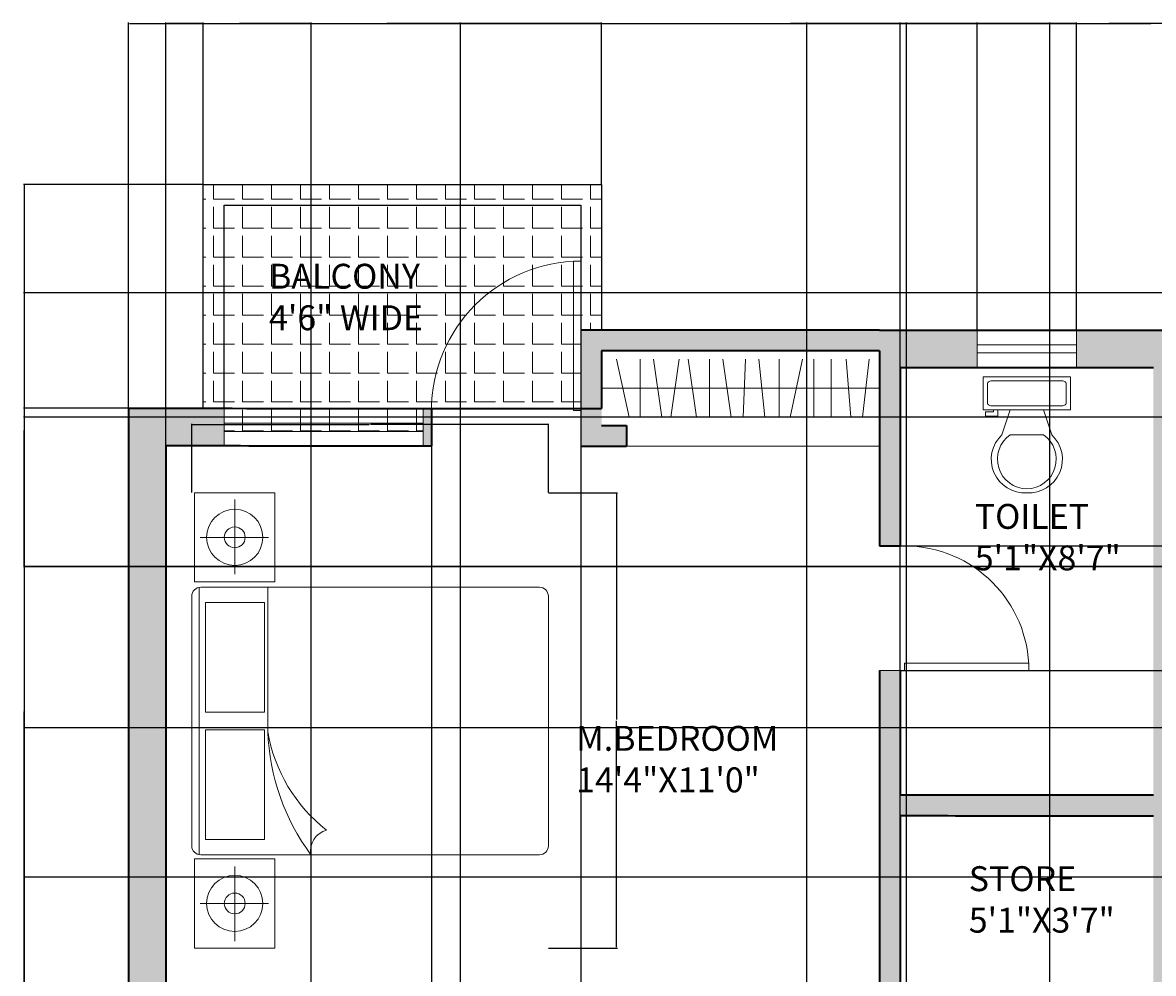
# Model space of a CAD drawing. Units: inches. Extents: x 1044 to 1567, y 918 to 1417.
# Tile 2 of 4: x 1044 to 1316, y 1148 to 1377. Entities that reach past the tile are written whole.
import ezdxf

# ---------------------------------------------------------------- set-up
doc = ezdxf.new("R2010")
doc.units = ezdxf.units.IN
for name, color, linetype, lineweight in [('A-ANNO-DIMS', 2, 'Continuous', 18), ('A-AREA-IDEN', 7, 'Continuous', 18), ('A-FLOR', 7, 'Continuous', 13), ('A-FLOR-CASE', 8, 'Continuous', 18), ('A-FLOR-FIXT', 9, 'Continuous', 18), ('A-FLOR-PATT', 9, 'Continuous', 13), ('A-FURN', 8, 'Continuous', 18), ('A-GLAZ', 4, 'Continuous', 13), ('A-WALL', 7, 'Continuous', 35), ('A-WALL-PATT', 252, 'Continuous', 13), ('A-WALL-PRPT', 7, 'Continuous', 25), ('door', 4, 'Continuous', 18)]:
    doc.layers.add(name, color=color, linetype=linetype, lineweight=lineweight)
doc.styles.get("Standard").update_dxf_attribs({"font": 'arial.ttf'})
doc.dimstyles.get("Standard").update_dxf_attribs({"dimtxt": 0.18, "dimasz": 0.18, "dimexe": 0.18, "dimexo": 0.0625, "dimgap": 0.09, "dimtad": 0, "dimtih": 1, "dimtoh": 1, "dimdec": 4, "dimzin": 0, "dimdsep": 46, "dimtxsty": 'Standard', "dimcen": 0.09, "dimadec": 0, "dimazin": 0, "dimtfac": 1, "dimtdec": 4, "dimtofl": 0, "dimtmove": 0, "dimatfit": 3, "dimfxl": 1, "dimtolj": 1, "dimtzin": 0, "dimarcsym": 0})
pattern_1 = [(0, (0, 0), (0, 6.985), [5.08, -1.905]), (90, (0, 0), (-6.985, 4e-16), [5.08, -1.905])]

# ---------------------------------------------------------------- blocks, each defined once
blk = doc.blocks.new('*U3')
for p, q in [((-30, 0), (-30, -6)), ((0, 0), (0, -6))]:
    blk.add_line(p, q)
blk.add_lwpolyline([(0, 0), (0, 30), (-1.75, 30), (-1.75, 0)], close=True)
blk.add_arc((0, 0), 30, 90, 180)
blk = doc.blocks.new('*U6')
for p, q in [((0, 0), (0, -6)), ((-36, 0), (-36, -6))]:
    blk.add_line(p, q)
blk.add_lwpolyline([(0, 0), (0, 36), (-1.75, 36), (-1.75, 0)], close=True)
blk.add_arc((0, 0), 36, 90, 180)
blk = doc.blocks.new('A$C3C75334F')
for p, q in [((0, 1.534), (0, 1.984)), ((0, 1.984), (0.5, 1.984)), ((0.5, 1.984), (0.5, 1.534)), ((1.9728, 2), (0.5728, 2)), ((2.0529, 1.984), (2.0529, 1.534)), ((2.5529, 1.984), (2.0529, 1.984)), ((2.5529, 1.534), (2.5529, 1.984)), ((0.25, 1.9525), (0.25, 1.57)), ((2.0228, 1.958), (0.5228, 1.958)), ((0.5228, 1.95), (0.5228, 0.05)), ((0.6089, 1.9225), (0.6089, 1.5925)), ((1.2239, 1.9225), (0.6089, 1.9225)), ((1.2239, 1.5925), (1.2239, 1.9225)), ((1.3217, 1.5925), (1.3217, 1.9225)), ((1.3217, 1.9225), (1.9367, 1.9225)), ((1.9367, 1.9225), (1.9367, 1.5925)), ((2.0228, 0.05), (2.0228, 1.95)), ((2.3029, 1.9525), (2.3029, 1.57)), ((0.457, 1.759), (0.0385, 1.759)), ((2.0959, 1.759), (2.5144, 1.759)), ((0.6089, 1.5925), (1.2239, 1.5925)), ((1.9367, 1.5925), (1.3217, 1.5925)), ((0.5, 1.534), (0, 1.534)), ((1.2128, 1.5739), (2.0228, 1.5739)), ((2.0529, 1.534), (2.5529, 1.534)), ((0.5728, 0), (1.9728, 0))]:
    blk.add_line(p, q)
for centre, radius in [((0.25, 1.759), 0.1575), ((2.3029, 1.759), 0.1575), ((0.25, 1.759), 0.0585), ((2.3029, 1.759), 0.0585)]:
    blk.add_circle(centre, radius)
for centre, radius, start, end in [((0.5728, 1.95), 0.05, 90, 180), ((1.9728, 1.95), 0.05, 0, 90), ((1.2652, 0.3179), 1.2571, 92.38351, 126.19807), ((1.3644, 0.6928), 0.894, 99.75657, 141.93721), ((0.544, 1.2137), 0.1205, 14.54629, 100.1199), ((0.5728, 0.05), 0.05, 180, 270), ((1.9728, 0.05), 0.05, 270, 0)]:
    blk.add_arc(centre, radius, start, end)
blk = doc.blocks.new('*U14')
for p, q in [((9.5, -6), (9.5, -2)), ((-8, -8.5), (-8, -8)), ((-7, -8), (-7, -9.5)), ((-4, -8), (-6, -14)), ((4, -8), (6, -14)), ((-10, -8.5), (-8, -8.5)), ((-10, -9.5), (-10, -8.5)), ((-7, -9.5), (-10, -9.5)), ((4, -14), (-4, -14))]:
    blk.add_line(p, q)
blk.add_lwpolyline([(10.5, -8), (10.5, 0), (-10.5, 0), (-10.5, -8)], close=True)
for points in [[(-9.5, -2), (-9.5, -6)], [(8.5, -1), (-8.5, -1)], [(-8.5, -7), (8.5, -7)]]:
    blk.add_lwpolyline(points)
for centre, radius, start, end in [((-8.625, -1.875), 0.8839, 81.8699, 188.1301), ((8.625, -1.875), 0.8839, 351.8699, 98.1301), ((-8.625, -6.125), 0.8839, 171.869898, 278.1301), ((8.625, -6.125), 0.8839, 261.8699, 8.1301), ((-0.4772, -19.9188), 8.0953, 133.01722, 273.38), ((0.0374, -19.8731), 7.127, 124.50543, 269.7), ((-0.0373, -19.8731), 7.127, 270.3, 55.4946), ((0.4773, -19.9188), 8.0953, 266.62, 46.9828)]:
    blk.add_arc(centre, radius, start, end)
blk = doc.blocks.new('GLAZ-PANEL-48IN')
for p, q in [((48, 2), (0, 2)), ((48, 0), (0, 0))]:
    blk.add_line(p, q)
blk = doc.blocks.new('*D16')
at = {"layer": 'A-ANNO-DIMS', "color": 0, "lineweight": -2, "transparency": 16777216}
for p, q in [((1170.41, 1263.37), (1186.99, 1263.37)), ((1186.81, 1263.19), (1186.81, 1208.7)), ((1186.81, 1153.84), (1186.81, 1208.33)), ((1170.41, 1153.66), (1186.99, 1153.66))]:
    blk.add_line(p, q, dxfattribs=at)
at = {"layer": 'A-ANNO-DIMS', "color": 0, "transparency": 16777216}
for points in [[(1186.78, 1263.19), (1186.84, 1263.19), (1186.81, 1263.37)], [(1186.78, 1153.84), (1186.84, 1153.84), (1186.81, 1153.66)]]:
    blk.add_solid(points, dxfattribs=at)
at = {"layer": 'Defpoints', "color": 0, "transparency": 16777216}
for p in [(1170.35, 1263.37), (1186.81, 1263.37), (1170.35, 1153.66)]:
    blk.add_point(p, dxfattribs=at)
at = {"layer": 'A-ANNO-DIMS', "color": 0, "transparency": 16777216, "insert": (1186.81, 1208.52), "char_height": 0.18, "attachment_point": 5}
blk.add_mtext('\\A1;BED GROUP 110', dxfattribs=at)
blk = doc.blocks.new('*D17')
at = {"layer": 'A-ANNO-DIMS', "color": 0, "lineweight": -2, "transparency": 16777216}
for p, q in [((1084.4, 1263.43), (1084.4, 1280.01)), ((1084.58, 1279.83), (1127.16, 1279.83)), ((1170.17, 1279.83), (1127.6, 1279.83)), ((1170.35, 1263.43), (1170.35, 1280.01))]:
    blk.add_line(p, q, dxfattribs=at)
at = {"layer": 'A-ANNO-DIMS', "color": 0, "transparency": 16777216}
for points in [[(1084.58, 1279.86), (1084.58, 1279.8), (1084.4, 1279.83)], [(1170.17, 1279.86), (1170.17, 1279.8), (1170.35, 1279.83)]]:
    blk.add_solid(points, dxfattribs=at)
at = {"layer": 'Defpoints', "color": 0, "transparency": 16777216}
for p in [(1084.4, 1279.83), (1084.4, 1263.37), (1170.35, 1263.37)]:
    blk.add_point(p, dxfattribs=at)
at = {"layer": 'A-ANNO-DIMS', "color": 0, "transparency": 16777216, "insert": (1127.38, 1279.83), "char_height": 0.18, "attachment_point": 5}
blk.add_mtext('\\A1;86', dxfattribs=at)
blk = doc.blocks.new('*D30')
at = {"layer": 'A-ANNO-DIMS', "color": 0, "lineweight": -2, "transparency": 16777216}
for p, q in [((1069.18, 1283.83), (1069.18, 1376.67)), ((1069.36, 1376.49), (1304.89, 1376.49)), ((1541, 1376.49), (1305.47, 1376.49)), ((1541.18, 1316.83), (1541.18, 1376.67))]:
    blk.add_line(p, q, dxfattribs=at)
at = {"layer": 'A-ANNO-DIMS', "color": 0, "transparency": 16777216}
for points in [[(1069.36, 1376.52), (1069.36, 1376.46), (1069.18, 1376.49)], [(1541, 1376.52), (1541, 1376.46), (1541.18, 1376.49)]]:
    blk.add_solid(points, dxfattribs=at)
at = {"layer": 'Defpoints', "color": 0, "transparency": 16777216}
for p in [(1541.18, 1376.49), (1541.18, 1316.77), (1069.18, 1283.77)]:
    blk.add_point(p, dxfattribs=at)
at = {"layer": 'A-ANNO-DIMS', "color": 0, "transparency": 16777216, "insert": (1305.18, 1376.49), "char_height": 0.18, "attachment_point": 5}
blk.add_mtext('\\A1;472', dxfattribs=at)
blk = doc.blocks.new('*D31')
at = {"layer": 'A-ANNO-DIMS', "color": 0, "lineweight": -2, "transparency": 16777216}
for p, q in [((1087.11, 1337.65), (1043.83, 1337.65)), ((1044.01, 1337.47), (1044.01, 1140.89)), ((1044.01, 943.95), (1044.01, 1140.53)), ((1069.11, 943.77), (1043.83, 943.77))]:
    blk.add_line(p, q, dxfattribs=at)
at = {"layer": 'A-ANNO-DIMS', "color": 0, "transparency": 16777216}
for points in [[(1043.98, 1337.47), (1044.04, 1337.47), (1044.01, 1337.65)], [(1043.98, 943.95), (1044.04, 943.95), (1044.01, 943.77)]]:
    blk.add_solid(points, dxfattribs=at)
at = {"layer": 'Defpoints', "color": 0, "transparency": 16777216}
for p in [(1044.01, 1337.65), (1087.18, 1337.65), (1069.18, 943.77)]:
    blk.add_point(p, dxfattribs=at)
at = {"layer": 'A-ANNO-DIMS', "color": 0, "transparency": 16777216, "insert": (1044.01, 1140.71), "char_height": 0.18, "attachment_point": 5}
blk.add_mtext('\\A1;393.9', dxfattribs=at)
blk = doc.blocks.new('*D40')
at = {"layer": 'A-ANNO-DIMS', "color": 0, "lineweight": -2, "transparency": 16777216}
for p, q in [((1069.18, 1283.83), (1069.18, 1376.67)), ((1069.36, 1376.49), (1077.97, 1376.49)), ((1087, 1376.49), (1078.39, 1376.49)), ((1087.18, 1337.72), (1087.18, 1376.67))]:
    blk.add_line(p, q, dxfattribs=at)
at = {"layer": 'A-ANNO-DIMS', "color": 0, "transparency": 16777216}
for points in [[(1069.36, 1376.52), (1069.36, 1376.46), (1069.18, 1376.49)], [(1087, 1376.52), (1087, 1376.46), (1087.18, 1376.49)]]:
    blk.add_solid(points, dxfattribs=at)
at = {"layer": 'Defpoints', "color": 0, "transparency": 16777216}
for p in [(1087.18, 1376.49), (1087.18, 1337.65), (1069.18, 1283.77)]:
    blk.add_point(p, dxfattribs=at)
at = {"layer": 'A-ANNO-DIMS', "color": 0, "transparency": 16777216, "insert": (1078.18, 1376.49), "char_height": 0.18, "attachment_point": 5}
blk.add_mtext('\\A1;18', dxfattribs=at)
blk = doc.blocks.new('*D41')
at = {"layer": 'A-ANNO-DIMS', "color": 0, "lineweight": -2, "transparency": 16777216}
for p, q in [((1087.18, 1337.72), (1087.18, 1376.67)), ((1087.36, 1376.49), (1134.96, 1376.49)), ((1183, 1376.49), (1135.4, 1376.49)), ((1183.18, 1337.72), (1183.18, 1376.67))]:
    blk.add_line(p, q, dxfattribs=at)
at = {"layer": 'A-ANNO-DIMS', "color": 0, "transparency": 16777216}
for points in [[(1087.36, 1376.52), (1087.36, 1376.46), (1087.18, 1376.49)], [(1183, 1376.52), (1183, 1376.46), (1183.18, 1376.49)]]:
    blk.add_solid(points, dxfattribs=at)
at = {"layer": 'Defpoints', "color": 0, "transparency": 16777216}
for p in [(1183.18, 1376.49), (1087.18, 1337.65), (1183.18, 1337.65)]:
    blk.add_point(p, dxfattribs=at)
at = {"layer": 'A-ANNO-DIMS', "color": 0, "transparency": 16777216, "insert": (1135.18, 1376.49), "char_height": 0.18, "attachment_point": 5}
blk.add_mtext('\\A1;96', dxfattribs=at)
blk = doc.blocks.new('*D42')
at = {"layer": 'A-ANNO-DIMS', "color": 0, "lineweight": -2, "transparency": 16777216}
for p, q in [((1183.18, 1337.72), (1183.18, 1376.67)), ((1183.36, 1376.49), (1228.1, 1376.49)), ((1273.5, 1376.49), (1228.75, 1376.49)), ((1273.68, 1302.62), (1273.68, 1376.67))]:
    blk.add_line(p, q, dxfattribs=at)
at = {"layer": 'A-ANNO-DIMS', "color": 0, "transparency": 16777216}
for points in [[(1183.36, 1376.52), (1183.36, 1376.46), (1183.18, 1376.49)], [(1273.5, 1376.52), (1273.5, 1376.46), (1273.68, 1376.49)]]:
    blk.add_solid(points, dxfattribs=at)
at = {"layer": 'Defpoints', "color": 0, "transparency": 16777216}
for p in [(1273.68, 1376.49), (1183.18, 1337.65), (1273.68, 1302.56)]:
    blk.add_point(p, dxfattribs=at)
at = {"layer": 'A-ANNO-DIMS', "color": 0, "transparency": 16777216, "insert": (1228.43, 1376.49), "char_height": 0.18, "attachment_point": 5}
blk.add_mtext('\\A1;90.5', dxfattribs=at)
blk = doc.blocks.new('*D43')
at = {"layer": 'A-ANNO-DIMS', "color": 0, "lineweight": -2, "transparency": 16777216}
for p, q in [((1273.68, 1302.62), (1273.68, 1376.67)), ((1273.86, 1376.49), (1285.46, 1376.49)), ((1297.5, 1376.49), (1285.9, 1376.49)), ((1297.68, 1302.62), (1297.68, 1376.67))]:
    blk.add_line(p, q, dxfattribs=at)
at = {"layer": 'A-ANNO-DIMS', "color": 0, "transparency": 16777216}
for points in [[(1273.86, 1376.52), (1273.86, 1376.46), (1273.68, 1376.49)], [(1297.5, 1376.52), (1297.5, 1376.46), (1297.68, 1376.49)]]:
    blk.add_solid(points, dxfattribs=at)
at = {"layer": 'Defpoints', "color": 0, "transparency": 16777216}
for p in [(1297.68, 1376.49), (1273.68, 1302.56), (1297.68, 1302.55)]:
    blk.add_point(p, dxfattribs=at)
at = {"layer": 'A-ANNO-DIMS', "color": 0, "transparency": 16777216, "insert": (1285.68, 1376.49), "char_height": 0.18, "attachment_point": 5}
blk.add_mtext('\\A1;24', dxfattribs=at)
blk = doc.blocks.new('*D44')
at = {"layer": 'A-ANNO-DIMS', "color": 0, "lineweight": -2, "transparency": 16777216}
for p, q in [((1297.68, 1302.62), (1297.68, 1376.67)), ((1297.86, 1376.49), (1315.6, 1376.49)), ((1334, 1376.49), (1316.25, 1376.49)), ((1334.18, 1316.62), (1334.18, 1376.67))]:
    blk.add_line(p, q, dxfattribs=at)
at = {"layer": 'A-ANNO-DIMS', "color": 0, "transparency": 16777216}
for points in [[(1297.86, 1376.52), (1297.86, 1376.46), (1297.68, 1376.49)], [(1334, 1376.52), (1334, 1376.46), (1334.18, 1376.49)]]:
    blk.add_solid(points, dxfattribs=at)
at = {"layer": 'Defpoints', "color": 0, "transparency": 16777216}
for p in [(1334.18, 1376.49), (1334.18, 1316.55), (1297.68, 1302.55)]:
    blk.add_point(p, dxfattribs=at)
at = {"layer": 'A-ANNO-DIMS', "color": 0, "transparency": 16777216, "insert": (1315.93, 1376.49), "char_height": 0.18, "attachment_point": 5}
blk.add_mtext('\\A1;36.5', dxfattribs=at)
blk = doc.blocks.new('*D47')
at = {"layer": 'A-ANNO-DIMS', "color": 0, "lineweight": -2, "transparency": 16777216}
for p, q in [((1069.11, 1283.77), (1043.83, 1283.77)), ((1044.01, 1283.59), (1044.01, 1210.94)), ((1044.01, 1137.93), (1044.01, 1210.58)), ((1078.11, 1137.75), (1043.83, 1137.75))]:
    blk.add_line(p, q, dxfattribs=at)
at = {"layer": 'A-ANNO-DIMS', "color": 0, "transparency": 16777216}
for points in [[(1043.98, 1283.59), (1044.04, 1283.59), (1044.01, 1283.77)], [(1043.98, 1137.93), (1044.04, 1137.93), (1044.01, 1137.75)]]:
    blk.add_solid(points, dxfattribs=at)
at = {"layer": 'Defpoints', "color": 0, "transparency": 16777216}
for p in [(1044.01, 1283.77), (1069.18, 1283.77), (1078.18, 1137.75)]:
    blk.add_point(p, dxfattribs=at)
at = {"layer": 'A-ANNO-DIMS', "color": 0, "transparency": 16777216, "insert": (1044.01, 1210.76), "char_height": 0.18, "attachment_point": 5}
blk.add_mtext('\\A1;146.02', dxfattribs=at)
blk = doc.blocks.new('*D48')
at = {"layer": 'A-ANNO-DIMS', "color": 0, "lineweight": -2, "transparency": 16777216}
for p, q in [((1142.18, 1274.59), (1142.18, 918.44)), ((1178.18, 1274.55), (1178.18, 918.44)), ((1142.36, 918.62), (1159.96, 918.62)), ((1178, 918.62), (1160.4, 918.62))]:
    blk.add_line(p, q, dxfattribs=at)
at = {"layer": 'A-ANNO-DIMS', "color": 0, "transparency": 16777216}
for points in [[(1142.36, 918.65), (1142.36, 918.59), (1142.18, 918.62)], [(1178, 918.65), (1178, 918.59), (1178.18, 918.62)]]:
    blk.add_solid(points, dxfattribs=at)
at = {"layer": 'Defpoints', "color": 0, "transparency": 16777216}
for p in [(1142.18, 1274.65), (1178.18, 1274.61), (1178.18, 918.62)]:
    blk.add_point(p, dxfattribs=at)
at = {"layer": 'A-ANNO-DIMS', "color": 0, "transparency": 16777216, "insert": (1160.18, 918.62), "char_height": 0.18, "attachment_point": 5}
blk.add_mtext('\\A1;36', dxfattribs=at)
blk = doc.blocks.new('*D49')
at = {"layer": 'A-ANNO-DIMS', "color": 0, "lineweight": -2, "transparency": 16777216}
for p, q in [((1078.18, 1002.26), (1078.18, 1376.67)), ((1078.36, 1376.49), (1095.46, 1376.49)), ((1113, 1376.49), (1095.9, 1376.49)), ((1113.18, 1001.71), (1113.18, 1376.67))]:
    blk.add_line(p, q, dxfattribs=at)
at = {"layer": 'A-ANNO-DIMS', "color": 0, "transparency": 16777216}
for points in [[(1078.36, 1376.52), (1078.36, 1376.46), (1078.18, 1376.49)], [(1113, 1376.52), (1113, 1376.46), (1113.18, 1376.49)]]:
    blk.add_solid(points, dxfattribs=at)
at = {"layer": 'Defpoints', "color": 0, "transparency": 16777216}
for p in [(1113.18, 1376.49), (1078.18, 1002.19), (1113.18, 1001.65)]:
    blk.add_point(p, dxfattribs=at)
at = {"layer": 'A-ANNO-DIMS', "color": 0, "transparency": 16777216, "insert": (1095.68, 1376.49), "char_height": 0.18, "attachment_point": 5}
blk.add_mtext('\\A1;35', dxfattribs=at)
blk = doc.blocks.new('*D50')
at = {"layer": 'A-ANNO-DIMS', "color": 0, "lineweight": -2, "transparency": 16777216}
for p, q in [((1113.18, 1001.71), (1113.18, 1376.67)), ((1113.36, 1376.49), (1130.96, 1376.49)), ((1149, 1376.49), (1131.4, 1376.49)), ((1149.18, 1001.71), (1149.18, 1376.67))]:
    blk.add_line(p, q, dxfattribs=at)
at = {"layer": 'A-ANNO-DIMS', "color": 0, "transparency": 16777216}
for points in [[(1113.36, 1376.52), (1113.36, 1376.46), (1113.18, 1376.49)], [(1149, 1376.52), (1149, 1376.46), (1149.18, 1376.49)]]:
    blk.add_solid(points, dxfattribs=at)
at = {"layer": 'Defpoints', "color": 0, "transparency": 16777216}
for p in [(1149.18, 1376.49), (1113.18, 1001.65), (1149.18, 1001.65)]:
    blk.add_point(p, dxfattribs=at)
at = {"layer": 'A-ANNO-DIMS', "color": 0, "transparency": 16777216, "insert": (1131.18, 1376.49), "char_height": 0.18, "attachment_point": 5}
blk.add_mtext('\\A1;36', dxfattribs=at)
blk = doc.blocks.new('*D51')
at = {"layer": 'A-ANNO-DIMS', "color": 0, "lineweight": -2, "transparency": 16777216}
for p, q in [((1443.11, 1206.74), (1043.83, 1206.74)), ((1044.01, 1206.56), (1044.01, 1188.92)), ((1044.01, 1170.92), (1044.01, 1188.56)), ((1443.11, 1170.74), (1043.83, 1170.74))]:
    blk.add_line(p, q, dxfattribs=at)
at = {"layer": 'A-ANNO-DIMS', "color": 0, "transparency": 16777216}
for points in [[(1043.98, 1206.56), (1044.04, 1206.56), (1044.01, 1206.74)], [(1043.98, 1170.92), (1044.04, 1170.92), (1044.01, 1170.74)]]:
    blk.add_solid(points, dxfattribs=at)
at = {"layer": 'Defpoints', "color": 0, "transparency": 16777216}
for p in [(1044.01, 1206.74), (1443.18, 1206.74), (1443.18, 1170.74)]:
    blk.add_point(p, dxfattribs=at)
at = {"layer": 'A-ANNO-DIMS', "color": 0, "transparency": 16777216, "insert": (1044.01, 1188.74), "char_height": 0.18, "attachment_point": 5}
blk.add_mtext('\\A1;36', dxfattribs=at)
blk = doc.blocks.new('*D53')
at = {"layer": 'A-ANNO-DIMS', "color": 0, "lineweight": -2, "transparency": 16777216}
for p, q in [((1255.24, 1250.56), (1566.52, 1250.56)), ((1566.34, 1250.38), (1566.34, 1235.74)), ((1566.34, 1220.74), (1566.34, 1235.38)), ((1255.24, 1220.56), (1566.52, 1220.56))]:
    blk.add_line(p, q, dxfattribs=at)
at = {"layer": 'A-ANNO-DIMS', "color": 0, "transparency": 16777216}
for points in [[(1566.31, 1250.38), (1566.37, 1250.38), (1566.34, 1250.56)], [(1566.31, 1220.74), (1566.37, 1220.74), (1566.34, 1220.56)]]:
    blk.add_solid(points, dxfattribs=at)
at = {"layer": 'Defpoints', "color": 0, "transparency": 16777216}
for p in [(1255.18, 1250.56), (1566.34, 1250.56), (1255.18, 1220.56)]:
    blk.add_point(p, dxfattribs=at)
at = {"layer": 'A-ANNO-DIMS', "color": 0, "transparency": 16777216, "insert": (1566.34, 1235.56), "char_height": 0.18, "attachment_point": 5}
blk.add_mtext('\\A1;30', dxfattribs=at)
blk = doc.blocks.new('*D57')
at = {"layer": 'A-ANNO-DIMS', "color": 0, "lineweight": -2, "transparency": 16777216}
for p, q in [((1255.18, 1137.62), (1255.18, 1376.67)), ((1255.36, 1376.49), (1272.96, 1376.49)), ((1291, 1376.49), (1273.4, 1376.49)), ((1291.18, 1142.61), (1291.18, 1376.67))]:
    blk.add_line(p, q, dxfattribs=at)
at = {"layer": 'A-ANNO-DIMS', "color": 0, "transparency": 16777216}
for points in [[(1255.36, 1376.52), (1255.36, 1376.46), (1255.18, 1376.49)], [(1291, 1376.52), (1291, 1376.46), (1291.18, 1376.49)]]:
    blk.add_solid(points, dxfattribs=at)
at = {"layer": 'Defpoints', "color": 0, "transparency": 16777216}
for p in [(1291.18, 1376.49), (1291.18, 1142.55), (1255.18, 1137.56)]:
    blk.add_point(p, dxfattribs=at)
at = {"layer": 'A-ANNO-DIMS', "color": 0, "transparency": 16777216, "insert": (1273.18, 1376.49), "char_height": 0.18, "attachment_point": 5}
blk.add_mtext('\\A1;36', dxfattribs=at)
blk = doc.blocks.new('*D60')
at = {"layer": 'A-ANNO-DIMS', "color": 0, "lineweight": -2, "transparency": 16777216}
for p, q in [((1443.11, 1281.62), (1043.83, 1281.62)), ((1044.01, 1281.44), (1044.01, 1263.79)), ((1044.01, 1245.78), (1044.01, 1263.43)), ((1443.15, 1245.6), (1043.83, 1245.6))]:
    blk.add_line(p, q, dxfattribs=at)
at = {"layer": 'A-ANNO-DIMS', "color": 0, "transparency": 16777216}
for points in [[(1043.98, 1281.44), (1044.04, 1281.44), (1044.01, 1281.62)], [(1043.98, 1245.78), (1044.04, 1245.78), (1044.01, 1245.6)]]:
    blk.add_solid(points, dxfattribs=at)
at = {"layer": 'Defpoints', "color": 0, "transparency": 16777216}
for p in [(1044.01, 1281.62), (1443.18, 1281.62), (1443.22, 1245.6)]:
    blk.add_point(p, dxfattribs=at)
at = {"layer": 'A-ANNO-DIMS', "color": 0, "transparency": 16777216, "insert": (1044.01, 1263.61), "char_height": 0.18, "attachment_point": 5}
blk.add_mtext('\\A1;36.03', dxfattribs=at)
blk = doc.blocks.new('*D61')
at = {"layer": 'A-ANNO-DIMS', "color": 0, "lineweight": -2, "transparency": 16777216}
for p, q in [((1339.11, 1311.56), (1043.83, 1311.56)), ((1044.01, 1311.38), (1044.01, 1278.74)), ((1044.01, 1245.74), (1044.01, 1278.37)), ((1339.11, 1245.56), (1043.83, 1245.56))]:
    blk.add_line(p, q, dxfattribs=at)
at = {"layer": 'A-ANNO-DIMS', "color": 0, "transparency": 16777216}
for points in [[(1043.98, 1311.38), (1044.04, 1311.38), (1044.01, 1311.56)], [(1043.98, 1245.74), (1044.04, 1245.74), (1044.01, 1245.56)]]:
    blk.add_solid(points, dxfattribs=at)
at = {"layer": 'Defpoints', "color": 0, "transparency": 16777216}
for p in [(1044.01, 1311.56), (1339.18, 1311.56), (1339.18, 1245.56)]:
    blk.add_point(p, dxfattribs=at)
at = {"layer": 'A-ANNO-DIMS', "color": 0, "transparency": 16777216, "insert": (1044.01, 1278.56), "char_height": 0.18, "attachment_point": 5}
blk.add_mtext('\\A1;66', dxfattribs=at)
blk = doc.blocks.new('*D62')
at = {"layer": 'A-ANNO-DIMS', "color": 0, "lineweight": -2, "transparency": 16777216}
for p, q in [((1232.68, 1001.63), (1232.68, 1376.67)), ((1232.86, 1376.49), (1244.46, 1376.49)), ((1256.5, 1376.49), (1244.9, 1376.49)), ((1256.68, 1001.62), (1256.68, 1376.67))]:
    blk.add_line(p, q, dxfattribs=at)
at = {"layer": 'A-ANNO-DIMS', "color": 0, "transparency": 16777216}
for points in [[(1232.86, 1376.52), (1232.86, 1376.46), (1232.68, 1376.49)], [(1256.5, 1376.52), (1256.5, 1376.46), (1256.68, 1376.49)]]:
    blk.add_solid(points, dxfattribs=at)
at = {"layer": 'Defpoints', "color": 0, "transparency": 16777216}
for p in [(1256.68, 1376.49), (1232.68, 1001.57), (1256.68, 1001.56)]:
    blk.add_point(p, dxfattribs=at)
at = {"layer": 'A-ANNO-DIMS', "color": 0, "transparency": 16777216, "insert": (1244.68, 1376.49), "char_height": 0.18, "attachment_point": 5}
blk.add_mtext('\\A1;24', dxfattribs=at)

msp = doc.modelspace()

# ---------------------------------------------------------------- hatches: boundary and pattern name
at = {"layer": 'A-FLOR-PATT'}
h = msp.add_hatch(dxfattribs=at)
h.set_pattern_fill('ANGLE', color=256)
h.set_pattern_definition(pattern_1)
h.paths.add_polyline_path([(1142.177, 1283.654, -0.0000039), (1140.177, 1283.657), (1140.177, 1278.134), (1092.177, 1278.134), (1092.177, 1283.727, -0.0000097), (1087.177, 1283.735), (1087.177, 1337.654), (1183.177, 1337.654), (1183.177, 1302.563), (1178.177, 1302.563), (1178.177, 1283.654)])
h.paths.add_polyline_path([(1321.177, 1245.553), (1327.676, 1269.552), (1321.174, 1293.553, 0.0000348), (1339.177, 1293.556), (1339.177, 1302.556, -0.0000097), (1334.177, 1302.555), (1334.177, 1316.555, 0.0002109), (1443.177, 1316.625), (1443.177, 1307.625, 0.0000445), (1466.198, 1307.652), (1457.182, 1298.636), (1466.177, 1289.652, -0.0000445), (1443.177, 1289.625), (1443.177, 1281.625), (1443.215, 1245.625, -0.0000465), (1419.177, 1245.602), (1419.177, 1240.063), (1377.177, 1240.063), (1377.177, 1245.572, -0.0000039), (1375.177, 1245.571), (1339.177, 1245.556, -0.0000348)])
h = msp.add_hatch(dxfattribs=at)
h.set_pattern_fill('ANGLE', color=256)
h.set_pattern_definition(pattern_1)
h.paths.add_polyline_path([(1178.177, 1332.654), (1092.177, 1332.654), (1092.177, 1283.726, 0.0003861), (1178.177, 1283.654)])
at = {"layer": 'A-WALL-PATT'}
h = msp.add_hatch(color=256, dxfattribs=at)
h.dxf.hatch_style = 1
h.paths.add_polyline_path([(1273.677, 1302.555, -0.0000455), (1250.177, 1302.563), (1178.177, 1302.563), (1178.177, 1274.614, 0.0000213), (1189.177, 1274.604), (1189.177, 1279.604, -0.0000116), (1183.177, 1279.609), (1183.177, 1297.563), (1250.177, 1297.563), (1250.177, 1250.563, 0.0000097), (1255.177, 1250.561), (1255.177, 1293.561, 0.0000358), (1273.677, 1293.555)])
h.paths.add_polyline_path([(1339.177, 1302.556, -0.0000348), (1321.176, 1302.553, -0.0000455), (1297.677, 1302.552), (1297.677, 1293.552, 0.0000358), (1316.177, 1293.552), (1316.177, 1190.552, -0.0001179), (1255.177, 1190.561), (1255.177, 1220.561, -0.0000097), (1250.177, 1220.563), (1250.177, 1137.563, 0.0000097), (1255.177, 1137.561), (1255.177, 1185.561, 0.0001179), (1316.177, 1185.552), (1316.177, 1142.552, -0.0000483), (1291.177, 1142.552), (1291.177, 1137.552, 0.000058), (1321.177, 1137.553), (1321.177, 1236.553, 0.0000348), (1339.177, 1236.556), (1339.177, 1245.556, -0.0000348), (1321.177, 1245.553), (1321.177, 1293.544), (1321.174, 1293.553, 0.0000348), (1339.177, 1293.556)])
h = msp.add_hatch(color=256, dxfattribs=at)
h.dxf.hatch_style = 1
h.paths.add_polyline_path([(1092.177, 1283.727, -0.0000445), (1069.177, 1283.767), (1069.177, 996.767, 0.0000174), (1078.177, 996.751), (1078.177, 1137.751, 0.0002628), (1214.177, 1137.584), (1214.177, 1142.584, -0.0002628), (1078.177, 1142.751), (1078.177, 1274.751, 0.0000271), (1092.177, 1274.727)])
h = msp.add_hatch(color=256, dxfattribs=at)
h.dxf.hatch_style = 1
h.paths.add_polyline_path([(1140.177, 1274.657, 0.0000038), (1142.165, 1274.654), (1142.177, 1283.668, -0.000009), (1140.177, 1283.669)])

# ---------------------------------------------------------------- linework, layer by layer
at = {"layer": 'A-FLOR'}
msp.add_arc((1305.177, 130508.416), 129287.864, 269.97562596, 270.00487368, dxfattribs=at)
at = {"layer": 'A-FLOR-CASE'}
for p, q in [((1186.813, 1295.563), (1189.812, 1281.603)), ((1192.494, 1295.563), (1192.494, 1281.601)), ((1197.699, 1281.596), (1195.657, 1295.563)), ((1201.845, 1295.563), (1199.845, 1281.594)), ((1204.029, 1295.563), (1206.057, 1281.59)), ((1209.224, 1295.563), (1209.224, 1281.587)), ((1212.408, 1295.563), (1214.437, 1281.583)), ((1217.296, 1281.581), (1217.874, 1295.563)), ((1221.069, 1295.563), (1222.497, 1281.578)), ((1225.954, 1295.563), (1225.954, 1281.576)), ((1231.585, 1295.563), (1228.642, 1281.574)), ((1234.319, 1295.563), (1234.319, 1281.571)), ((1238.502, 1295.563), (1238.502, 1281.569)), ((1242.094, 1295.563), (1243.278, 1281.566)), ((1246.049, 1281.565), (1247.657, 1295.563)), ((1183.177, 1288.586), (1250.177, 1288.586)), ((1189.177, 1274.604), (1250.177, 1274.604))]:
    msp.add_line(p, q, dxfattribs=at)
at = {"layer": 'A-GLAZ'}
for p, q in [((1273.677, 1293.553), (1273.677, 1302.555)), ((1297.677, 1293.552), (1297.677, 1302.553)), ((1297.677, 1299.053), (1273.677, 1299.053)), ((1297.677, 1297.053), (1273.677, 1297.053)), ((1092.177, 1283.654), (1092.177, 1274.614)), ((1140.177, 1283.654), (1140.177, 1274.614))]:
    msp.add_line(p, q, dxfattribs=at)
at = {"layer": 'A-WALL'}
for p, q in [((1250.177, 1302.563), (1178.177, 1302.563)), ((1250.177, 1297.563), (1183.177, 1297.563)), ((1183.177, 1297.563), (1183.177, 1283.654)), ((1250.177, 1297.563), (1250.177, 1250.563)), ((1255.177, 1293.561), (1255.177, 1250.561)), ((1069.177, 1283.767), (1069.177, 996.767)), ((1142.177, 1283.654), (1142.165, 1274.654)), ((1189.177, 1279.604), (1189.177, 1274.604)), ((1078.177, 1274.751), (1078.177, 1142.751)), ((1250.177, 1220.563), (1250.177, 1137.563)), ((1255.177, 1220.561), (1255.177, 1190.561)), ((1255.177, 1185.561), (1255.177, 1137.561))]:
    msp.add_line(p, q, dxfattribs=at)
for centre, radius, start, end in [((1305.177, 130508.416), 129205.864, 269.97561049, 270.00709513), ((1305.177, 130508.416), 129214.864, 269.97782926, 270.00487756), ((1181.241, 56963.22), 55679.566, 269.8846831, 270.0019922), ((1305.177, 130520.416), 129240.864, 269.94591427, 269.94857423), ((1305.177, 130520.416), 129245.864, 269.89537187, 269.89537916), ((1305.177, 130520.416), 129245.864, 269.89936894, 269.92774071), ((1305.177, 130520.416), 129245.864, 269.94369982, 269.94857622), ((1305.177, 130508.416), 129257.864, 269.9756203, 269.97783664), ((1305.177, 130508.416), 129317.864, 269.97784692, 270.00487368), ((1305.177, 130508.416), 129322.864, 269.97784778, 270.00487349)]:
    msp.add_arc(centre, radius, start, end, dxfattribs=at)
at = {"layer": 'A-WALL-PRPT'}
for p, q in [((1087.177, 1337.654), (1183.177, 1337.654)), ((1087.177, 1283.654), (1087.177, 1337.654)), ((1183.177, 1337.654), (1183.177, 1302.563)), ((1092.177, 1283.654), (1092.177, 1332.654)), ((1092.177, 1332.654), (1178.177, 1332.654)), ((1178.177, 1332.654), (1178.177, 1274.614))]:
    msp.add_line(p, q, dxfattribs=at)

# ---------------------------------------------------------------- block references
at = {"layer": 'A-FLOR-FIXT'}
msp.add_blockref('*U14', (1285.677, 1291.336), dxfattribs=at)
at = {"layer": 'A-FURN', "xscale": 42.97459308160635, "yscale": 42.97459308160635, "zscale": 42.97459308160635, "rotation": 90}
msp.add_blockref('A$C3C75334F', (1170.352, 1153.663), dxfattribs=at)
at = {"layer": 'A-GLAZ'}
msp.add_blockref('GLAZ-PANEL-48IN', (1092.177, 1278.134), dxfattribs=at)
at = {"layer": 'door'}
msp.add_blockref('*U6', (1178.177, 1283.184), dxfattribs=at)
at = {"layer": 'door', "rotation": 270}
msp.add_blockref('*U3', (1256.177, 1220.563), dxfattribs=at)

# ---------------------------------------------------------------- texts
at = {"layer": 'A-AREA-IDEN', "char_height": 6, "attachment_point": 1}
for s, insert in [('BALCONY\\P4\'6" WIDE', (1103.031, 1318.548)), ('TOILET\\P5\'1"X8\'7"', (1273.132, 1260.675)), ('M.BEDROOM\\P14\'4"X11\'0"', (1177.056, 1207.186)), ('STORE\\P5\'1"X3\'7"', (1271.677, 1173.374))]:
    msp.add_mtext_dynamic_manual_height_columns(s, width=56.12489, gutter_width=12.5, heights=[0], dxfattribs=dict(at, insert=insert))

# ---------------------------------------------------------------- dimensions: what is measured, and where the dimension line sits
at = {"layer": 'A-ANNO-DIMS'}
for base, p1, p2, override, picture, middle in [((1541.177, 1376.486), (1069.177, 1283.767), (1541.177, 1316.767), {"dimdec": 0, "dimlfac": 1, "dimrnd": 0, "dimzin": 0, "dimdsep": 46, "dimlunit": 2}, '*D30', (1305.177, 1376.486)), ((1087.177, 1376.486), (1069.177, 1283.767), (1087.177, 1337.654), {"dimdec": 0, "dimlfac": 1, "dimrnd": 0, "dimzin": 0, "dimdsep": 46, "dimlunit": 2}, '*D40', (1078.177, 1376.486)), ((1113.177, 1376.486), (1078.177, 1002.194), (1113.177, 1001.646), {"dimdec": 0, "dimlfac": 1, "dimrnd": 0, "dimzin": 0, "dimdsep": 46, "dimlunit": 2}, '*D49', (1095.677, 1376.486)), ((1183.177, 1376.486), (1087.177, 1337.654), (1183.177, 1337.654), {"dimdec": 0, "dimlfac": 1, "dimrnd": 0, "dimzin": 0, "dimdsep": 46, "dimlunit": 2}, '*D41', (1135.177, 1376.486)), ((1149.177, 1376.486), (1113.177, 1001.646), (1149.177, 1001.646), {"dimdec": 0, "dimlfac": 1, "dimrnd": 0, "dimzin": 0, "dimdsep": 46, "dimlunit": 2}, '*D50', (1131.177, 1376.486)), ((1273.677, 1376.486), (1183.177, 1337.654), (1273.677, 1302.555), {"dimdec": 1, "dimlfac": 1, "dimrnd": 0, "dimzin": 0, "dimdsep": 46, "dimlunit": 2}, '*D42', (1228.427, 1376.486)), ((1256.677, 1376.486), (1232.677, 1001.571), (1256.677, 1001.56), {"dimdec": 0, "dimlfac": 1, "dimrnd": 0, "dimzin": 0, "dimdsep": 46, "dimlunit": 2}, '*D62', (1244.677, 1376.486)), ((1291.177, 1376.486), (1255.177, 1137.561), (1291.177, 1142.552), {"dimdec": 0, "dimlfac": 1, "dimrnd": 0, "dimzin": 0, "dimdsep": 46, "dimlunit": 2}, '*D57', (1273.177, 1376.486)), ((1297.677, 1376.486), (1273.677, 1302.555), (1297.677, 1302.553), {"dimdec": 0, "dimlfac": 1, "dimrnd": 0, "dimzin": 0, "dimdsep": 46, "dimlunit": 2}, '*D43', (1285.677, 1376.486)), ((1334.177, 1376.486), (1297.677, 1302.553), (1334.177, 1316.555), {"dimdec": 1, "dimlfac": 1, "dimrnd": 0, "dimzin": 0, "dimdsep": 46, "dimlunit": 2}, '*D44', (1315.927, 1376.486)), ((1178.177, 918.617), (1142.177, 1274.654), (1178.177, 1274.614), {"dimdec": 0, "dimlfac": 1, "dimrnd": 0, "dimzin": 0, "dimdsep": 46, "dimlunit": 2}, '*D48', (1160.177, 918.617))]:
    dim = msp.add_linear_dim(base=base, p1=p1, p2=p2, dimstyle='Standard', override=override, dxfattribs=at)
    dim.commit()
    dim.dimension.update_dxf_attribs({"geometry": picture, "text_midpoint": middle})
for base, p1, p2, angle, override, picture, middle in [((1044.01, 1337.654), (1069.177, 943.767), (1087.177, 1337.654), 90, {"dimdec": 1, "dimlfac": 1, "dimrnd": 0, "dimzin": 0, "dimdsep": 46, "dimlunit": 2}, '*D31', (1044.01, 1140.71)), ((1044.01, 1311.556), (1339.177, 1245.556), (1339.177, 1311.556), 90, {"dimdec": 0, "dimlfac": 1, "dimrnd": 0, "dimzin": 0, "dimdsep": 46, "dimlunit": 2}, '*D61', (1044.01, 1278.556)), ((1044.01, 1283.767), (1078.177, 1137.751), (1069.177, 1283.767), 90, {"dimdec": 2, "dimlfac": 1, "dimrnd": 0, "dimzin": 0, "dimdsep": 46, "dimlunit": 2}, '*D47', (1044.01, 1210.759)), ((1044.01, 1281.625), (1443.215, 1245.598), (1443.177, 1281.625), 90, {"dimdec": 2, "dimlfac": 1, "dimrnd": 0, "dimzin": 0, "dimdsep": 46, "dimlunit": 2}, '*D60', (1044.01, 1263.611)), ((1084.402, 1279.829), (1170.352, 1263.372), (1084.402, 1263.372), 180, {"dimdec": 0, "dimlfac": 1, "dimrnd": 0, "dimzin": 0, "dimdsep": 46, "dimlunit": 2}, '*D17', (1127.377, 1279.829)), ((1566.336, 1250.561), (1255.177, 1220.561), (1255.177, 1250.561), 90, {"dimdec": 0, "dimlfac": 1, "dimrnd": 0, "dimzin": 0, "dimdsep": 46, "dimlunit": 2}, '*D53', (1566.336, 1235.561)), ((1044.01, 1206.739), (1443.177, 1170.739), (1443.177, 1206.739), 90, {"dimdec": 0, "dimlfac": 1, "dimrnd": 0, "dimzin": 0, "dimdsep": 46, "dimlunit": 2}, '*D51', (1044.01, 1188.739))]:
    dim = msp.add_linear_dim(base=base, p1=p1, p2=p2, angle=angle, dimstyle='Standard', override=override, dxfattribs=at)
    dim.commit()
    dim.dimension.update_dxf_attribs({"geometry": picture, "text_midpoint": middle})
dim = msp.add_linear_dim(base=(1186.808, 1263.372), p1=(1170.352, 1153.663), p2=(1170.352, 1263.372), angle=90, text='BED GROUP <>', dimstyle='Standard', override={"dimdec": 0, "dimlfac": 1, "dimrnd": 0, "dimzin": 0, "dimdsep": 46, "dimlunit": 2}, dxfattribs=at)
dim.commit()
dim.dimension.update_dxf_attribs({"geometry": '*D16', "text_midpoint": (1186.808, 1208.518)})

doc.saveas('drawing.dxf')
